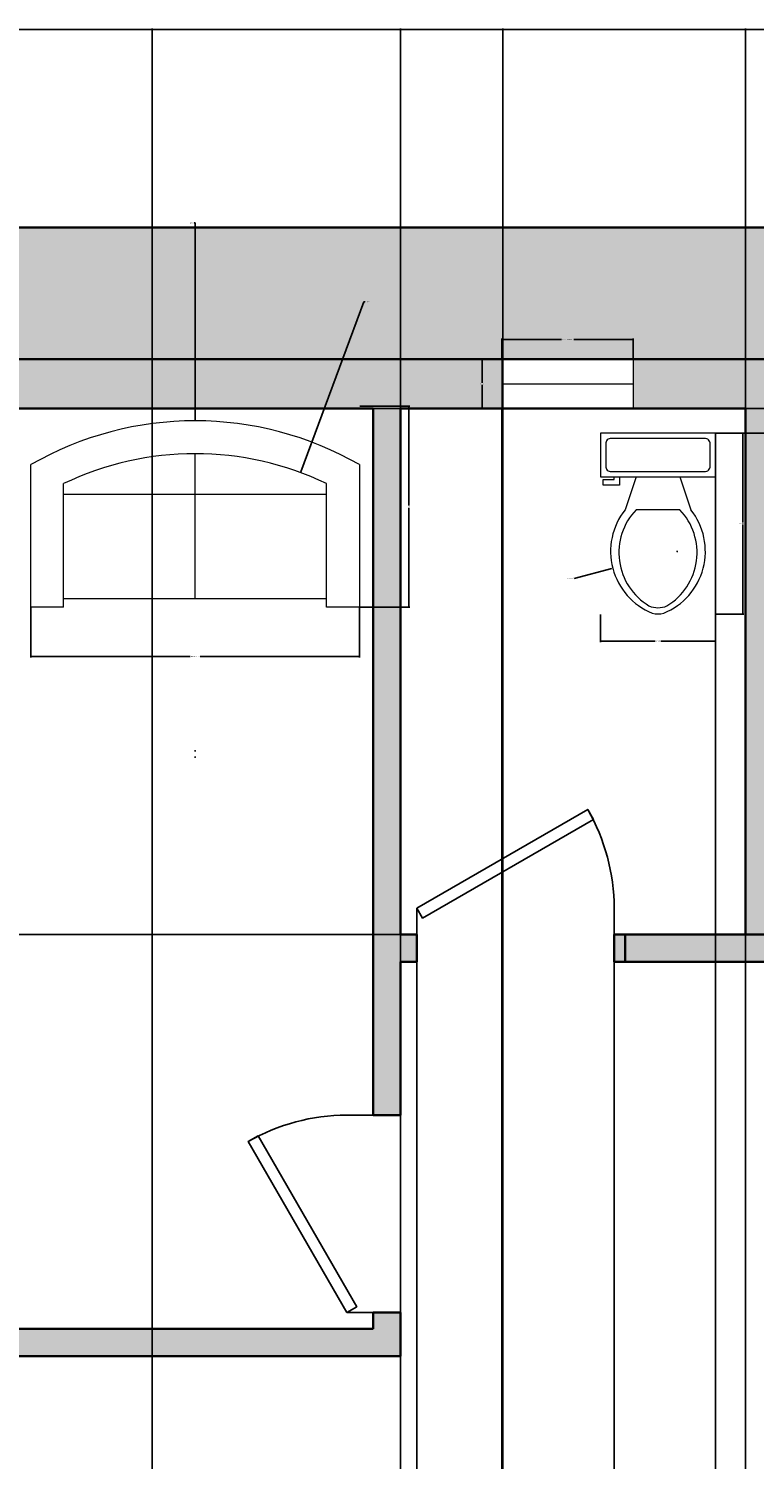
# Model space of a CAD drawing. Units: inches. Extents: x -7 to 546, y -27 to 766.
# Tile 7 of 9: x 143 to 276, y 505 to 766. Entities that reach past the tile are written whole.
import ezdxf

# ---------------------------------------------------------------- set-up
doc = ezdxf.new("R2010")
doc.units = ezdxf.units.IN
doc.header["$MEASUREMENT"] = 0
for name, color, linetype, lineweight in [('A-ANNO-DIMS', 2, 'Continuous', 18), ('A-FLOR-FIXT', 9, 'Continuous', 18), ('A-WALL', 7, 'Continuous', 35), ('C-PROP', 7, 'Continuous', 35), ('doors', 40, 'Continuous', 25), ('furniture', 220, 'Continuous', 18), ('window', 30, 'Continuous', 20)]:
    doc.layers.add(name, color=color, linetype=linetype, lineweight=lineweight)
doc.layers.add('A-WALL-PATT', color=251, linetype='Continuous', lineweight=13, true_color=0x636466)
doc.layers.add('L-PLNT-PATT', color=85, linetype='Continuous', lineweight=13, true_color=0x58ba48)
doc.styles.get("Standard").update_dxf_attribs({"font": 'arial.ttf'})
doc.dimstyles.get("Standard").update_dxf_attribs({"dimtxt": 0.18, "dimasz": 0.18, "dimexe": 0.18, "dimexo": 0.0625, "dimgap": 0.09, "dimtad": 0, "dimtih": 1, "dimtoh": 1, "dimdec": 4, "dimzin": 0, "dimdsep": 46, "dimtxsty": 'Standard', "dimcen": 0.09, "dimadec": 0, "dimazin": 0, "dimtfac": 1, "dimtdec": 4, "dimtofl": 0, "dimtmove": 0, "dimatfit": 3, "dimfxl": 1, "dimtolj": 1, "dimtzin": 0, "dimarcsym": 0})

# ---------------------------------------------------------------- blocks, each defined once
blk = doc.blocks.new('*U10')
for p, q in [((0, 0), (0, -100)), ((750, 0), (750, -100))]:
    blk.add_line(p, q)
blk.add_lwpolyline([(0, 0), (649.5, 375), (671.4, 337.1), (21.9, -37.9)], close=True)
blk.add_arc((0, 0), 750, 0, 30)
blk = doc.blocks.new('Sofa - Roundback Loveseat 5 ft.')
for p, q in [((0, -32.44198), (0, -5.99998)), ((-24, -33.99998), (-24, -11.46958)), ((24.00004, -33.99998), (24.00004, -11.46958)), ((-23.9998, -13.38178), (23.99986, -13.38178)), ((-24, -32.44198), (24.00004, -32.44198))]:
    blk.add_line(p, q)
for points in [[(-24, -33.99998), (-30, -33.99998), (-30, -7.99998)], [(30.00004, -7.99998), (30.00004, -33.99998), (24.00004, -33.99998)]]:
    blk.add_lwpolyline(points)
for centre, radius, start, end in [((0, -60.24998), 60.24998, 60.13715, 119.8628), ((0, -61.38438), 55.38444, 64.32083, 115.6792)]:
    blk.add_arc(centre, radius, start, end)
blk = doc.blocks.new('Toilet - top')
for p, q in [((9.5, -6), (9.5, -2)), ((-10, -8.5), (-8, -8.5)), ((-10, -9.5), (-10, -8.5)), ((-7, -9.5), (-10, -9.5)), ((-8, -8.5), (-8, -8)), ((-7, -8), (-7, -9.5)), ((-4, -8), (-6, -14)), ((4, -8), (6, -14)), ((4, -14), (-4, -14))]:
    blk.add_line(p, q)
blk.add_lwpolyline([(10.5, -8), (10.5, 0), (-10.5, 0), (-10.5, -8)], close=True)
for points in [[(-9.5, -2), (-9.5, -6)], [(8.5, -1), (-8.5, -1)], [(-8.5, -7), (8.5, -7)]]:
    blk.add_lwpolyline(points)
for centre, radius, start, end in [((-8.62, -1.88), 0.884, 81.8699, 188.1301), ((8.62, -1.88), 0.884, 351.8699, 98.1301), ((-8.62, -6.12), 0.884, 171.8699, 278.1301), ((8.62, -6.12), 0.884, 261.8699, 8.1301), ((3.52, -21.58), 12.17, 141.4691, 247.9714), ((4.2, -21.82), 11.33, 136.3677, 238.9468), ((-3.52, -21.58), 12.17, 292.0284, 38.5307), ((-4.2, -21.82), 11.33, 301.053, 43.6321), ((0, -27.88), 4, 245.7318, 294.2682), ((0, -29), 4, 254.8605, 285.1395)]:
    blk.add_arc(centre, radius, start, end)
blk = doc.blocks.new('WIN-24IN')
for p, q in [((0, 9), (0, 0)), ((24, 9), (0, 9)), ((0, 9), (0, 4.5)), ((24, 0), (24, 9)), ((0, 4.5), (24, 4.5)), ((0, 0), (24, 0))]:
    blk.add_line(p, q)
blk = doc.blocks.new('*D16')
at = {"layer": 'A-ANNO-DIMS', "color": 0, "lineweight": -2, "transparency": 16777216}
for p, q in [((229.74, 705.81), (229.74, 709.52)), ((229.92, 709.34), (240.62, 709.34)), ((253.56, 709.34), (242.86, 709.34)), ((253.74, 705.81), (253.74, 709.52))]:
    blk.add_line(p, q, dxfattribs=at)
at = {"layer": 'A-ANNO-DIMS', "color": 0, "transparency": 16777216}
for points in [[(229.92, 709.37), (229.92, 709.31), (229.74, 709.34)], [(253.56, 709.37), (253.56, 709.31), (253.74, 709.34)]]:
    blk.add_solid(points, dxfattribs=at)
at = {"layer": 'Defpoints', "color": 0, "transparency": 16777216}
for p in [(253.74, 709.34), (229.74, 705.74), (253.74, 705.74)]:
    blk.add_point(p, dxfattribs=at)
at = {"layer": 'A-ANNO-DIMS', "color": 0, "transparency": 16777216, "insert": (241.74, 709.34), "char_height": 0.18, "attachment_point": 5}
blk.add_mtext('\\A1;WINDOW 24 TYP.', dxfattribs=at)
blk = doc.blocks.new('*D17')
at = {"layer": 'A-ANNO-DIMS', "color": 0, "lineweight": -2, "transparency": 16777216}
for p, q in [((229.68, 705.74), (225.96, 705.74)), ((226.14, 705.56), (226.14, 701.43)), ((226.14, 696.92), (226.14, 701.06)), ((229.68, 696.74), (225.96, 696.74))]:
    blk.add_line(p, q, dxfattribs=at)
at = {"layer": 'A-ANNO-DIMS', "color": 0, "transparency": 16777216}
for points in [[(226.11, 705.56), (226.17, 705.56), (226.14, 705.74)], [(226.11, 696.92), (226.17, 696.92), (226.14, 696.74)]]:
    blk.add_solid(points, dxfattribs=at)
at = {"layer": 'Defpoints', "color": 0, "transparency": 16777216}
for p in [(226.14, 705.74), (229.74, 705.74), (229.74, 696.74)]:
    blk.add_point(p, dxfattribs=at)
at = {"layer": 'A-ANNO-DIMS', "color": 0, "transparency": 16777216, "insert": (226.14, 701.24), "char_height": 0.18, "attachment_point": 5}
blk.add_mtext('\\A1;9 TYP.', dxfattribs=at)
blk = doc.blocks.new('*D22')
at = {"layer": 'A-ANNO-DIMS', "color": 0, "lineweight": -2, "transparency": 16777216}
for p, q in [((143.76, 660.41), (143.76, 651.29)), ((203.76, 660.41), (203.76, 651.29)), ((143.94, 651.47), (172.85, 651.47)), ((203.58, 651.47), (174.67, 651.47))]:
    blk.add_line(p, q, dxfattribs=at)
at = {"layer": 'A-ANNO-DIMS', "color": 0, "transparency": 16777216}
for points in [[(143.94, 651.5), (143.94, 651.44), (143.76, 651.47)], [(203.58, 651.5), (203.58, 651.44), (203.76, 651.47)]]:
    blk.add_solid(points, dxfattribs=at)
at = {"layer": 'Defpoints', "color": 0, "transparency": 16777216}
for p in [(143.76, 660.47), (203.76, 660.47), (203.76, 651.47)]:
    blk.add_point(p, dxfattribs=at)
at = {"layer": 'A-ANNO-DIMS', "color": 0, "transparency": 16777216, "insert": (173.76, 651.47), "char_height": 0.18, "attachment_point": 5}
blk.add_mtext('\\A1;LOVESEAT 60', dxfattribs=at)
blk = doc.blocks.new('*D23')
at = {"layer": 'A-ANNO-DIMS', "color": 0, "lineweight": -2, "transparency": 16777216}
for p, q in [((203.82, 697.14), (212.94, 697.14)), ((212.76, 696.96), (212.76, 678.99)), ((212.76, 660.65), (212.76, 678.62)), ((203.82, 660.47), (212.94, 660.47))]:
    blk.add_line(p, q, dxfattribs=at)
at = {"layer": 'A-ANNO-DIMS', "color": 0, "transparency": 16777216}
for points in [[(212.73, 696.96), (212.79, 696.96), (212.76, 697.14)], [(212.73, 660.65), (212.79, 660.65), (212.76, 660.47)]]:
    blk.add_solid(points, dxfattribs=at)
at = {"layer": 'Defpoints', "color": 0, "transparency": 16777216}
for p in [(203.76, 697.14), (212.76, 697.14), (203.76, 660.47)]:
    blk.add_point(p, dxfattribs=at)
at = {"layer": 'A-ANNO-DIMS', "color": 0, "transparency": 16777216, "insert": (212.76, 678.81), "char_height": 0.18, "attachment_point": 5}
blk.add_mtext('\\A1;37', dxfattribs=at)
blk = doc.blocks.new('*D28')
at = {"layer": 'A-ANNO-DIMS', "color": 0, "lineweight": -2, "transparency": 16777216}
for p, q in [((268.8, 692.23), (273.88, 692.23)), ((273.7, 692.05), (273.7, 675.89)), ((273.7, 659.37), (273.7, 675.53)), ((268.8, 659.19), (273.88, 659.19))]:
    blk.add_line(p, q, dxfattribs=at)
at = {"layer": 'A-ANNO-DIMS', "color": 0, "transparency": 16777216}
for points in [[(273.67, 692.05), (273.73, 692.05), (273.7, 692.23)], [(273.67, 659.37), (273.73, 659.37), (273.7, 659.19)]]:
    blk.add_solid(points, dxfattribs=at)
at = {"layer": 'Defpoints', "color": 0, "transparency": 16777216}
for p in [(268.74, 692.23), (273.7, 692.23), (268.74, 659.19)]:
    blk.add_point(p, dxfattribs=at)
at = {"layer": 'A-ANNO-DIMS', "color": 0, "transparency": 16777216, "insert": (273.7, 675.71), "char_height": 0.18, "attachment_point": 5}
blk.add_mtext('\\A1;WC 33 TYP.', dxfattribs=at)
blk = doc.blocks.new('*D29')
at = {"layer": 'A-ANNO-DIMS', "color": 0, "lineweight": -2, "transparency": 16777216}
for p, q in [((247.74, 659.12), (247.74, 654.05)), ((268.74, 659.12), (268.74, 654.05)), ((247.92, 654.23), (257.71, 654.23)), ((268.56, 654.23), (258.77, 654.23))]:
    blk.add_line(p, q, dxfattribs=at)
at = {"layer": 'A-ANNO-DIMS', "color": 0, "transparency": 16777216}
for points in [[(247.92, 654.26), (247.92, 654.2), (247.74, 654.23)], [(268.56, 654.26), (268.56, 654.2), (268.74, 654.23)]]:
    blk.add_solid(points, dxfattribs=at)
at = {"layer": 'Defpoints', "color": 0, "transparency": 16777216}
for p in [(247.74, 659.19), (268.74, 659.19), (268.74, 654.23)]:
    blk.add_point(p, dxfattribs=at)
at = {"layer": 'A-ANNO-DIMS', "color": 0, "transparency": 16777216, "insert": (258.24, 654.23), "char_height": 0.18, "attachment_point": 5}
blk.add_mtext('\\A1;21 TYP.', dxfattribs=at)
blk = doc.blocks.new('*D32')
at = {"layer": 'A-ANNO-DIMS', "color": 0, "lineweight": -2, "transparency": 16777216}
for p, q in [((53.23, 705.81), (53.23, 766.05)), ((53.41, 765.87), (268.94, 765.87)), ((485.05, 765.87), (269.52, 765.87)), ((485.23, 705.81), (485.23, 766.05))]:
    blk.add_line(p, q, dxfattribs=at)
at = {"layer": 'A-ANNO-DIMS', "color": 0, "transparency": 16777216}
for points in [[(53.41, 765.9), (53.41, 765.84), (53.23, 765.87)], [(485.05, 765.9), (485.05, 765.84), (485.23, 765.87)]]:
    blk.add_solid(points, dxfattribs=at)
at = {"layer": 'Defpoints', "color": 0, "transparency": 16777216}
for p in [(485.23, 765.87), (53.23, 705.74), (485.23, 705.74)]:
    blk.add_point(p, dxfattribs=at)
at = {"layer": 'A-ANNO-DIMS', "color": 0, "transparency": 16777216, "insert": (269.23, 765.87), "char_height": 0.18, "attachment_point": 5}
blk.add_mtext('\\A1;432', dxfattribs=at)
blk = doc.blocks.new('*D36')
at = {"layer": 'A-ANNO-DIMS', "color": 0, "lineweight": -2, "transparency": 16777216}
for p, q in [((211.23, 696.81), (211.23, 766.05)), ((211.41, 765.87), (242.51, 765.87)), ((274.05, 765.87), (242.95, 765.87)), ((274.23, 696.81), (274.23, 766.05))]:
    blk.add_line(p, q, dxfattribs=at)
at = {"layer": 'A-ANNO-DIMS', "color": 0, "transparency": 16777216}
for points in [[(211.41, 765.9), (211.41, 765.84), (211.23, 765.87)], [(274.05, 765.9), (274.05, 765.84), (274.23, 765.87)]]:
    blk.add_solid(points, dxfattribs=at)
at = {"layer": 'Defpoints', "color": 0, "transparency": 16777216}
for p in [(274.23, 765.87), (211.23, 696.74), (274.23, 696.74)]:
    blk.add_point(p, dxfattribs=at)
at = {"layer": 'A-ANNO-DIMS', "color": 0, "transparency": 16777216, "insert": (242.73, 765.87), "char_height": 0.18, "attachment_point": 5}
blk.add_mtext('\\A1;63', dxfattribs=at)
blk = doc.blocks.new('*D38')
at = {"layer": 'A-ANNO-DIMS', "color": 0, "lineweight": -2, "transparency": 16777216}
for p, q in [((211.17, 696.74), (-7.07, 696.74)), ((-6.89, 696.56), (-6.89, 648.93)), ((-6.89, 600.92), (-6.89, 648.56)), ((211.17, 600.74), (-7.07, 600.74))]:
    blk.add_line(p, q, dxfattribs=at)
at = {"layer": 'A-ANNO-DIMS', "color": 0, "transparency": 16777216}
for points in [[(-6.92, 696.56), (-6.86, 696.56), (-6.89, 696.74)], [(-6.92, 600.92), (-6.86, 600.92), (-6.89, 600.74)]]:
    blk.add_solid(points, dxfattribs=at)
at = {"layer": 'Defpoints', "color": 0, "transparency": 16777216}
for p in [(211.23, 696.74), (-6.89, 600.74), (211.23, 600.74)]:
    blk.add_point(p, dxfattribs=at)
at = {"layer": 'A-ANNO-DIMS', "color": 0, "transparency": 16777216, "insert": (-6.89, 648.74), "char_height": 0.18, "attachment_point": 5}
blk.add_mtext('\\A1;96', dxfattribs=at)
blk = doc.blocks.new('*D39')
at = {"layer": 'A-ANNO-DIMS', "color": 0, "lineweight": -2, "transparency": 16777216}
for p, q in [((214.23, 600.68), (214.23, -26.56)), ((250.23, 600.68), (250.23, -26.56)), ((214.41, -26.38), (232.01, -26.38)), ((250.05, -26.38), (232.45, -26.38))]:
    blk.add_line(p, q, dxfattribs=at)
at = {"layer": 'A-ANNO-DIMS', "color": 0, "transparency": 16777216}
for points in [[(214.41, -26.35), (214.41, -26.41), (214.23, -26.38)], [(250.05, -26.35), (250.05, -26.41), (250.23, -26.38)]]:
    blk.add_solid(points, dxfattribs=at)
at = {"layer": 'Defpoints', "color": 0, "transparency": 16777216}
for p in [(214.23, 600.74), (250.23, 600.74), (250.23, -26.38)]:
    blk.add_point(p, dxfattribs=at)
at = {"layer": 'A-ANNO-DIMS', "color": 0, "transparency": 16777216, "insert": (232.23, -26.38), "char_height": 0.18, "attachment_point": 5}
blk.add_mtext('\\A1;36', dxfattribs=at)
blk = doc.blocks.new('*D41')
at = {"layer": 'A-ANNO-DIMS', "color": 0, "lineweight": -2, "transparency": 16777216}
for p, q in [((274.23, 600.68), (274.23, -26.56)), ((279.23, 600.68), (279.23, -26.56)), ((274.41, -26.38), (276.58, -26.38)), ((279.05, -26.38), (276.88, -26.38))]:
    blk.add_line(p, q, dxfattribs=at)
at = {"layer": 'A-ANNO-DIMS', "color": 0, "transparency": 16777216}
for points in [[(274.41, -26.35), (274.41, -26.41), (274.23, -26.38)], [(279.05, -26.35), (279.05, -26.41), (279.23, -26.38)]]:
    blk.add_solid(points, dxfattribs=at)
at = {"layer": 'Defpoints', "color": 0, "transparency": 16777216}
for p in [(274.23, 600.74), (279.23, 600.74), (279.23, -26.38)]:
    blk.add_point(p, dxfattribs=at)
at = {"layer": 'A-ANNO-DIMS', "color": 0, "transparency": 16777216, "insert": (276.73, -26.38), "char_height": 0.18, "attachment_point": 5}
blk.add_mtext('\\A1;5', dxfattribs=at)
blk = doc.blocks.new('*D42')
at = {"layer": 'A-ANNO-DIMS', "color": 0, "lineweight": -2, "transparency": 16777216}
for p, q in [((211.23, 696.68), (211.23, -26.56)), ((229.74, 696.68), (229.74, -26.56)), ((211.41, -26.38), (220.12, -26.38)), ((229.56, -26.38), (220.85, -26.38))]:
    blk.add_line(p, q, dxfattribs=at)
at = {"layer": 'A-ANNO-DIMS', "color": 0, "transparency": 16777216}
for points in [[(211.41, -26.35), (211.41, -26.41), (211.23, -26.38)], [(229.56, -26.35), (229.56, -26.41), (229.74, -26.38)]]:
    blk.add_solid(points, dxfattribs=at)
at = {"layer": 'Defpoints', "color": 0, "transparency": 16777216}
for p in [(211.23, 696.74), (229.74, 696.74), (229.74, -26.38)]:
    blk.add_point(p, dxfattribs=at)
at = {"layer": 'A-ANNO-DIMS', "color": 0, "transparency": 16777216, "insert": (220.49, -26.38), "char_height": 0.18, "attachment_point": 5}
blk.add_mtext('\\A1;18.51', dxfattribs=at)
blk = doc.blocks.new('*D45')
at = {"layer": 'A-ANNO-DIMS', "color": 0, "lineweight": -2, "transparency": 16777216}
for p, q in [((211.23, 600.68), (211.23, -26.56)), ((214.23, 600.68), (214.23, -26.56)), ((211.41, -26.38), (212.58, -26.38)), ((214.05, -26.38), (212.88, -26.38))]:
    blk.add_line(p, q, dxfattribs=at)
at = {"layer": 'A-ANNO-DIMS', "color": 0, "transparency": 16777216}
for points in [[(211.41, -26.35), (211.41, -26.41), (211.23, -26.38)], [(214.05, -26.35), (214.05, -26.41), (214.23, -26.38)]]:
    blk.add_solid(points, dxfattribs=at)
at = {"layer": 'Defpoints', "color": 0, "transparency": 16777216}
for p in [(211.23, 600.74), (214.23, 600.74), (214.23, -26.38)]:
    blk.add_point(p, dxfattribs=at)
at = {"layer": 'A-ANNO-DIMS', "color": 0, "transparency": 16777216, "insert": (212.73, -26.38), "char_height": 0.18, "attachment_point": 5}
blk.add_mtext('\\A1;3', dxfattribs=at)
blk = doc.blocks.new('*D53')
at = {"layer": 'A-ANNO-DIMS', "color": 0, "lineweight": -2, "transparency": 16777216}
for p, q in [((133.93, 124.01), (133.93, 766.05)), ((134.11, 765.87), (181.71, 765.87)), ((229.75, 765.87), (182.15, 765.87)), ((229.93, 124.01), (229.93, 766.05))]:
    blk.add_line(p, q, dxfattribs=at)
at = {"layer": 'A-ANNO-DIMS', "color": 0, "transparency": 16777216}
for points in [[(134.11, 765.9), (134.11, 765.84), (133.93, 765.87)], [(229.75, 765.9), (229.75, 765.84), (229.93, 765.87)]]:
    blk.add_solid(points, dxfattribs=at)
at = {"layer": 'Defpoints', "color": 0, "transparency": 16777216}
for p in [(229.93, 765.87), (133.93, 123.94), (229.93, 123.94)]:
    blk.add_point(p, dxfattribs=at)
at = {"layer": 'A-ANNO-DIMS', "color": 0, "transparency": 16777216, "insert": (181.93, 765.87), "char_height": 0.18, "attachment_point": 5}
blk.add_mtext('\\A1;96', dxfattribs=at)
blk = doc.blocks.new('*D68')
at = {"layer": 'A-ANNO-DIMS', "color": 0, "lineweight": -2, "transparency": 16777216}
for p, q in [((133.93, 100.01), (133.93, 766.05)), ((134.11, 765.87), (149.71, 765.87)), ((165.75, 765.87), (150.15, 765.87)), ((165.93, 104.01), (165.93, 766.05))]:
    blk.add_line(p, q, dxfattribs=at)
at = {"layer": 'A-ANNO-DIMS', "color": 0, "transparency": 16777216}
for points in [[(134.11, 765.9), (134.11, 765.84), (133.93, 765.87)], [(165.75, 765.9), (165.75, 765.84), (165.93, 765.87)]]:
    blk.add_solid(points, dxfattribs=at)
at = {"layer": 'Defpoints', "color": 0, "transparency": 16777216}
for p in [(165.93, 765.87), (165.93, 103.94), (133.93, 99.94)]:
    blk.add_point(p, dxfattribs=at)
at = {"layer": 'A-ANNO-DIMS', "color": 0, "transparency": 16777216, "insert": (149.93, 765.87), "char_height": 0.18, "attachment_point": 5}
blk.add_mtext('\\A1;32', dxfattribs=at)
blk = doc.blocks.new('*D81')
at = {"layer": 'A-ANNO-DIMS', "color": 0, "lineweight": -2, "transparency": 16777216}
for p, q in [((62.23, 240.81), (62.23, 766.05)), ((62.41, 765.87), (194.44, 765.87)), ((327.05, 765.87), (195.02, 765.87)), ((327.23, 234.81), (327.23, 766.05))]:
    blk.add_line(p, q, dxfattribs=at)
at = {"layer": 'A-ANNO-DIMS', "color": 0, "transparency": 16777216}
for points in [[(62.41, 765.9), (62.41, 765.84), (62.23, 765.87)], [(327.05, 765.9), (327.05, 765.84), (327.23, 765.87)]]:
    blk.add_solid(points, dxfattribs=at)
at = {"layer": 'Defpoints', "color": 0, "transparency": 16777216}
for p in [(327.23, 765.87), (62.23, 240.74), (327.23, 234.74)]:
    blk.add_point(p, dxfattribs=at)
at = {"layer": 'A-ANNO-DIMS', "color": 0, "transparency": 16777216, "insert": (194.73, 765.87), "char_height": 0.18, "attachment_point": 5}
blk.add_mtext('\\A1;265', dxfattribs=at)
blk = doc.blocks.new('*D85')
at = {"layer": 'A-ANNO-DIMS', "color": 0, "lineweight": -2, "transparency": 16777216}
for p, q in [((274.23, 696.68), (274.23, -26.56)), ((268.74, 692.17), (268.74, -26.56)), ((268.92, -26.38), (271.09, -26.38)), ((274.05, -26.38), (271.88, -26.38))]:
    blk.add_line(p, q, dxfattribs=at)
at = {"layer": 'A-ANNO-DIMS', "color": 0, "transparency": 16777216}
for points in [[(268.92, -26.35), (268.92, -26.41), (268.74, -26.38)], [(274.05, -26.35), (274.05, -26.41), (274.23, -26.38)]]:
    blk.add_solid(points, dxfattribs=at)
at = {"layer": 'Defpoints', "color": 0, "transparency": 16777216}
for p in [(274.23, 696.74), (268.74, 692.23), (268.74, -26.38)]:
    blk.add_point(p, dxfattribs=at)
at = {"layer": 'A-ANNO-DIMS', "color": 0, "transparency": 16777216, "insert": (271.49, -26.38), "char_height": 0.18, "attachment_point": 5}
blk.add_mtext('\\A1;5.493', dxfattribs=at)
blk = doc.blocks.new('*D86')
at = {"layer": 'A-ANNO-DIMS', "color": 0, "lineweight": -2, "transparency": 16777216}
for p, q in [((274.29, 696.74), (545.54, 696.74)), ((545.36, 696.56), (545.36, 694.67)), ((268.8, 692.23), (545.54, 692.23)), ((545.36, 692.41), (545.36, 694.31))]:
    blk.add_line(p, q, dxfattribs=at)
at = {"layer": 'A-ANNO-DIMS', "color": 0, "transparency": 16777216}
for points in [[(545.33, 696.56), (545.39, 696.56), (545.36, 696.74)], [(545.33, 692.41), (545.39, 692.41), (545.36, 692.23)]]:
    blk.add_solid(points, dxfattribs=at)
at = {"layer": 'Defpoints', "color": 0, "transparency": 16777216}
for p in [(274.23, 696.74), (268.74, 692.23), (545.36, 692.23)]:
    blk.add_point(p, dxfattribs=at)
at = {"layer": 'A-ANNO-DIMS', "color": 0, "transparency": 16777216, "insert": (545.36, 694.49), "char_height": 0.18, "attachment_point": 5}
blk.add_mtext('\\A1;4.512', dxfattribs=at)
blk = doc.blocks.new('*D91')
at = {"layer": 'A-ANNO-DIMS', "color": 0, "lineweight": -2, "transparency": 16777216}
for p, q in [((173.58, 730.62), (173.76, 730.62)), ((173.76, 730.62), (173.76, 694.65)), ((173.67, 634.22), (173.85, 634.22)), ((173.76, 634.13), (173.76, 634.31))]:
    blk.add_line(p, q, dxfattribs=at)
at = {"layer": 'A-ANNO-DIMS', "color": 0, "transparency": 16777216}
blk.add_solid([(173.79, 694.65), (173.73, 694.65), (173.76, 694.47)], dxfattribs=at)
at = {"layer": 'Defpoints', "color": 0, "transparency": 16777216}
for p in [(173.76, 694.47), (173.76, 634.22)]:
    blk.add_point(p, dxfattribs=at)
at = {"layer": 'A-ANNO-DIMS', "color": 0, "transparency": 16777216, "insert": (173.1, 730.62), "char_height": 0.18, "attachment_point": 5}
blk.add_mtext('\\A1;R60.25', dxfattribs=at)
blk = doc.blocks.new('*D92')
at = {"layer": 'A-ANNO-DIMS', "color": 0, "lineweight": -2, "transparency": 16777216}
for p, q in [((204.55, 716.18), (193.06, 685.19)), ((204.73, 716.18), (204.55, 716.18)), ((173.67, 633.09), (173.85, 633.09)), ((173.76, 633), (173.76, 633.18))]:
    blk.add_line(p, q, dxfattribs=at)
at = {"layer": 'A-ANNO-DIMS', "color": 0, "transparency": 16777216}
blk.add_solid([(193.04, 685.2), (193.09, 685.18), (193, 685.02)], dxfattribs=at)
at = {"layer": 'Defpoints', "color": 0, "transparency": 16777216}
for p in [(193, 685.02), (173.76, 633.09)]:
    blk.add_point(p, dxfattribs=at)
at = {"layer": 'A-ANNO-DIMS', "color": 0, "transparency": 16777216, "insert": (205.21, 716.18), "char_height": 0.18, "attachment_point": 5}
blk.add_mtext('\\A1;R55.38', dxfattribs=at)
blk = doc.blocks.new('*D93')
at = {"layer": 'A-ANNO-DIMS', "color": 0, "lineweight": -2, "transparency": 16777216}
for p, q in [((261.67, 670.65), (261.85, 670.65)), ((261.76, 670.56), (261.76, 670.74)), ((242.93, 665.71), (249.81, 667.51))]:
    blk.add_line(p, q, dxfattribs=at)
at = {"layer": 'A-ANNO-DIMS', "color": 0, "transparency": 16777216}
blk.add_solid([(249.81, 667.54), (249.82, 667.49), (249.99, 667.56)], dxfattribs=at)
at = {"layer": 'Defpoints', "color": 0, "transparency": 16777216}
for p in [(261.76, 670.65), (249.99, 667.56)]:
    blk.add_point(p, dxfattribs=at)
at = {"layer": 'A-ANNO-DIMS', "color": 0, "transparency": 16777216, "insert": (242.25, 665.71), "char_height": 0.18, "attachment_point": 5}
blk.add_mtext('\\A1;6X R12.17', dxfattribs=at)

msp = doc.modelspace()

# ---------------------------------------------------------------- hatches: boundary and pattern name
at = {"layer": 'A-WALL-PATT'}
h = msp.add_hatch(color=256, dxfattribs=at)
h.dxf.hatch_style = 1
h.paths.add_polyline_path([(62.2319, 696.744), (86.6896, 696.744), (86.6896, 705.744), (53.2319, 705.744), (53.2319, 627.8642), (57.7271, 627.8642), (62.2319, 627.8642)])
h.paths.add_polyline_path([(229.7414, 705.744), (134.6896, 705.744), (134.6896, 696.744), (206.2319, 696.744), (206.2319, 567.744), (211.2319, 567.744), (211.2319, 595.744), (214.2319, 595.744), (214.2319, 600.744), (211.2319, 600.744), (211.2319, 696.744), (229.7414, 696.744)])
h.paths.add_polyline_path([(293.8423, 705.744), (253.7414, 705.744), (253.7414, 696.744), (274.2319, 696.744), (274.2319, 600.744), (279.2319, 600.744), (279.2319, 696.744), (293.8423, 696.744)])
h.paths.add_polyline_path([(393.9743, 705.744), (317.8423, 705.744), (317.8423, 696.744), (327.2319, 696.744), (327.2319, 651.744), (332.2319, 651.744), (332.2319, 696.744), (393.9743, 696.744)])
h.paths.add_polyline_path([(485.2319, 705.744), (441.9743, 705.744), (441.9743, 696.744), (476.2319, 696.744), (476.2319, 663.6898), (480.7319, 663.6898), (485.2319, 663.6898)])
h.paths.add_polyline_path([(485.2319, 615.6898), (476.2319, 615.6898), (476.2319, 528.744), (332.2319, 528.744), (332.2319, 531.744), (327.2319, 531.744), (327.2319, 523.744), (375.2319, 523.744), (375.2319, 427.744), (327.2319, 427.744), (327.2319, 419.744), (332.2319, 419.744), (332.2319, 422.744), (413.089, 422.744), (413.089, 427.744), (380.2319, 427.744), (380.2319, 523.744), (476.2319, 523.744), (476.2319, 490.9334), (485.2319, 490.9334)])
h.paths.add_polyline_path([(485.2319, 466.9334), (476.2319, 466.9334), (476.2319, 370.0932), (480.7319, 370.0932), (485.2319, 370.0932)])
h.paths.add_polyline_path([(485.2319, 322.0932), (476.2319, 322.0932), (476.2319, 278.744), (332.2319, 278.744), (332.2319, 383.744), (327.2319, 383.744), (327.2319, 273.744), (327.2319, 270.744), (332.2319, 270.744), (332.2319, 273.744), (476.2319, 273.744), (476.2319, 201.0338), (480.7319, 201.0338), (485.2319, 201.0338)])
h.paths.add_polyline_path([(485.2319, 153.0338), (476.2319, 153.0338), (476.2319, 42.744), (461.2319, 42.744), (461.2319, 33.744), (485.2319, 33.744)])
h.paths.add_polyline_path([(332.2319, 234.744), (327.2319, 234.744), (327.2319, 160.744), (315.2319, 160.744), (315.2319, 151.744), (327.2319, 151.744), (327.2319, 33.744), (332.2319, 33.744)])
h.paths.add_polyline_path([(252.2319, 151.744), (258.4464, 151.744), (264.2319, 151.744), (264.2319, 160.744), (252.2319, 160.744), (252.2319, 172.744), (247.2319, 172.744), (247.2319, 91.744), (127.2319, 91.744), (127.2319, 196.744), (122.2319, 196.744), (122.2319, 91.744), (62.2319, 91.744), (62.2319, 126.1124), (53.2319, 126.1124), (53.2319, 9.744), (62.2319, 9.744), (62.2319, 86.744), (247.2319, 86.744), (247.2319, 33.744), (252.2319, 33.744), (252.2319, 53.744)])
h.paths.add_polyline_path([(62.2319, 235.744), (122.2319, 235.744), (122.2319, 232.744), (127.2319, 232.744), (127.2319, 235.744), (247.2319, 235.744), (247.2319, 220.744), (252.2319, 220.744), (252.2319, 240.744), (250.6678, 240.744), (247.2319, 240.744), (62.2319, 240.744), (62.2319, 322.0932), (53.2319, 322.0932), (53.2319, 174.1124), (57.7271, 174.1124), (62.2319, 174.1124)])
h = msp.add_hatch(color=256, dxfattribs=at)
h.dxf.hatch_style = 1
h.paths.add_polyline_path([(327.2319, 600.744), (252.2319, 600.744), (252.2319, 595.744), (327.2319, 595.744)])
h.paths.add_polyline_path([(332.2319, 615.744), (327.2319, 615.744), (327.2319, 567.744), (332.2319, 567.744)])
h.paths.add_polyline_path([(252.2319, 600.744), (250.2319, 600.744), (250.2319, 595.744), (252.2319, 595.744)])
h = msp.add_hatch(color=256, dxfattribs=at)
h.dxf.hatch_style = 1
h.paths.add_polyline_path([(62.2319, 456.9275), (53.2319, 456.9275), (53.2319, 370.0932), (57.7271, 370.0932), (62.2319, 370.0932)])
h.paths.add_polyline_path([(62.2319, 579.8642), (53.2319, 579.8642), (53.2319, 504.9275), (57.7271, 504.9275), (62.2319, 504.9275), (62.2319, 523.744), (211.2319, 523.744), (211.2319, 531.744), (206.2319, 531.744), (206.2319, 528.744), (62.2319, 528.744)])
at = {"layer": 'L-PLNT-PATT'}
h = msp.add_hatch(color=256, dxfattribs=at)
h.dxf.hatch_style = 1
h.paths.add_polyline_path([(509.2319, 729.744), (29.2319, 729.744), (29.2319, 9.744), (53.2319, 9.744), (53.2319, 705.744), (485.2319, 705.744), (485.2319, 33.744), (461.2319, 33.744), (461.2319, 9.744), (509.2319, 9.744)])

# ---------------------------------------------------------------- linework, layer by layer
at = {"layer": 'A-WALL'}
for p, q in [((206.2319, 696.744), (62.2319, 696.744)), ((206.2319, 696.744), (206.2319, 567.744)), ((274.2319, 696.744), (211.2319, 696.744)), ((211.2319, 696.744), (211.2319, 600.744)), ((274.2319, 600.744), (274.2319, 696.744)), ((214.2319, 600.744), (211.2319, 600.744)), ((214.2319, 600.744), (214.2319, 595.744)), ((327.2319, 600.744), (250.2319, 600.744)), ((250.2319, 600.744), (250.2319, 595.744)), ((252.2319, 600.744), (252.2319, 595.744)), ((214.2319, 595.744), (211.2319, 595.744)), ((211.2319, 595.744), (211.2319, 567.744)), ((327.2319, 595.744), (250.2319, 595.744)), ((211.2319, 567.744), (206.2319, 567.744)), ((211.2319, 531.744), (206.2319, 531.744)), ((206.2319, 531.744), (206.2319, 528.744)), ((211.2319, 531.744), (211.2319, 523.744)), ((206.2319, 528.744), (62.2319, 528.744)), ((211.2319, 523.744), (62.2319, 523.744))]:
    msp.add_line(p, q, dxfattribs=at)
msp.add_lwpolyline([(461.2319, 33.744), (485.2319, 33.744), (485.2319, 705.744), (53.2319, 705.744), (53.2319, 9.744)], dxfattribs=at)
at = {"layer": 'C-PROP'}
msp.add_lwpolyline([(29.2319, 9.744), (509.2319, 9.744), (509.2319, 729.744), (29.2319, 729.744)], close=True, dxfattribs=at)

# ---------------------------------------------------------------- block references
at = {"layer": 'A-FLOR-FIXT'}
msp.add_blockref('Toilet - top', (258.2385, 692.2322), dxfattribs=at)
at = {"layer": 'doors', "xscale": 0.0480000000000013, "yscale": 0.0480000000000013, "zscale": 0.0480000000000013}
msp.add_blockref('*U10', (214.2319, 605.544), dxfattribs=at)
at = {"layer": 'doors', "xscale": 0.0480000000000013, "yscale": 0.0480000000000013, "zscale": 0.0480000000000013, "rotation": 90}
msp.add_blockref('*U10', (201.4319, 531.744), dxfattribs=at)
at = {"layer": 'furniture'}
msp.add_blockref('Sofa - Roundback Loveseat 5 ft.', (173.7595, 694.4717), dxfattribs=at)
at = {"layer": 'window'}
msp.add_blockref('WIN-24IN', (229.741, 696.744), dxfattribs=at)

# ---------------------------------------------------------------- dimensions: what is measured, and where the dimension line sits
at = {"layer": 'A-ANNO-DIMS'}
for base, p1, p2, override, picture, middle in [((485.2319, 765.869), (53.2319, 705.744), (485.2319, 705.744), {"dimdec": 0, "dimlfac": 1, "dimrnd": 0, "dimzin": 0, "dimdsep": 46, "dimlunit": 2}, '*D32', (269.2319, 765.869)), ((327.2319, 765.869), (62.2319, 240.744), (327.2319, 234.744), {"dimdec": 0, "dimlfac": 1, "dimrnd": 0, "dimzin": 0, "dimdsep": 46, "dimlunit": 2}, '*D81', (194.7319, 765.869)), ((229.9271, 765.869), (133.9271, 123.9426), (229.9271, 123.9426), {"dimdec": 0, "dimlfac": 1, "dimrnd": 0, "dimzin": 0, "dimdsep": 46, "dimlunit": 2}, '*D53', (181.9271, 765.869)), ((165.9271, 765.869), (133.9271, 99.9426), (165.9271, 103.9426), {"dimdec": 0, "dimlfac": 1, "dimrnd": 0, "dimzin": 0, "dimdsep": 46, "dimlunit": 2}, '*D68', (149.9271, 765.869)), ((274.2319, 765.869), (211.2319, 696.744), (274.2319, 696.744), {"dimdec": 0, "dimlfac": 1, "dimrnd": 0, "dimzin": 0, "dimdsep": 46, "dimlunit": 2}, '*D36', (242.7319, 765.869)), ((229.7414, -26.381), (211.2319, 696.744), (229.7414, 696.744), {"dimdec": 2, "dimlfac": 1, "dimrnd": 0, "dimzin": 0, "dimdsep": 46, "dimlunit": 2}, '*D42', (220.4867, -26.381)), ((268.7385, -26.381), (274.2319, 696.744), (268.7385, 692.2322), {"dimdec": 3, "dimlfac": 1, "dimrnd": 0, "dimzin": 0, "dimdsep": 46, "dimlunit": 2}, '*D85', (271.4852, -26.381)), ((214.2319, -26.381), (211.2319, 600.744), (214.2319, 600.744), {"dimdec": 0, "dimlfac": 1, "dimrnd": 0, "dimzin": 0, "dimdsep": 46, "dimlunit": 2}, '*D45', (212.7319, -26.381)), ((250.2319, -26.381), (214.2319, 600.744), (250.2319, 600.744), {"dimdec": 0, "dimlfac": 1, "dimrnd": 0, "dimzin": 0, "dimdsep": 46, "dimlunit": 2}, '*D39', (232.2319, -26.381)), ((279.2319, -26.381), (274.2319, 600.744), (279.2319, 600.744), {"dimdec": 0, "dimlfac": 1, "dimrnd": 0, "dimzin": 0, "dimdsep": 46, "dimlunit": 2}, '*D41', (276.7319, -26.381))]:
    dim = msp.add_linear_dim(base=base, p1=p1, p2=p2, dimstyle='Standard', override=override, dxfattribs=at)
    dim.commit()
    dim.dimension.update_dxf_attribs({"geometry": picture, "text_midpoint": middle})
for center, mpoint, picture, middle in [((173.7595, 634.2217), (173.759, 694.4717), '*D91', (173.0982, 730.6217)), ((173.7595, 633.0873), (193.0007, 685.022), '*D92', (205.2055, 716.1828))]:
    dim = msp.add_radius_dim(center=center, mpoint=mpoint, dimstyle='Standard', override={"dimdec": 2, "dimlfac": 1, "dimrnd": 0, "dimzin": 0, "dimdsep": 46, "dimlunit": 2}, dxfattribs=at)
    dim.commit()
    dim.dimension.update_dxf_attribs({"geometry": picture, "text_midpoint": middle, "dimtype": 164})
for base, p1, p2, text, picture, middle in [((253.7414, 709.344), (229.7414, 705.744), (253.7414, 705.744), 'WINDOW <> TYP.', '*D16', (241.7414, 709.344)), ((203.7595, 651.4717), (143.7595, 660.4717), (203.7595, 660.4717), 'LOVESEAT <>', '*D22', (173.7595, 651.4717)), ((268.7385, 654.229), (247.7385, 659.1859), (268.7385, 659.1859), '<> TYP.', '*D29', (258.2385, 654.229))]:
    dim = msp.add_linear_dim(base=base, p1=p1, p2=p2, text=text, dimstyle='Standard', override={"dimdec": 0, "dimlfac": 1, "dimrnd": 0, "dimzin": 0, "dimdsep": 46, "dimlunit": 2}, dxfattribs=at)
    dim.commit()
    dim.dimension.update_dxf_attribs({"geometry": picture, "text_midpoint": middle})
for base, p1, p2, text, picture, middle in [((226.1414, 705.744), (229.7414, 696.744), (229.7414, 705.744), '<> TYP.', '*D17', (226.1414, 701.244)), ((273.6954, 692.2322), (268.7385, 659.1859), (268.7385, 692.2322), 'WC <> TYP.', '*D28', (273.6954, 675.7091))]:
    dim = msp.add_linear_dim(base=base, p1=p1, p2=p2, angle=90, text=text, dimstyle='Standard', override={"dimdec": 0, "dimlfac": 1, "dimrnd": 0, "dimzin": 0, "dimdsep": 46, "dimlunit": 2}, dxfattribs=at)
    dim.commit()
    dim.dimension.update_dxf_attribs({"geometry": picture, "text_midpoint": middle})
for base, p1, p2, override, picture, middle in [((-6.8931, 600.744), (211.2319, 696.744), (211.2319, 600.744), {"dimdec": 0, "dimlfac": 1, "dimrnd": 0, "dimzin": 0, "dimdsep": 46, "dimlunit": 2}, '*D38', (-6.8931, 648.744)), ((212.7595, 697.1384), (203.7595, 660.4717), (203.7595, 697.1384), {"dimdec": 0, "dimlfac": 1, "dimrnd": 0, "dimzin": 0, "dimdsep": 46, "dimlunit": 2}, '*D23', (212.7595, 678.8051)), ((545.3569, 692.2322), (274.2319, 696.744), (268.7385, 692.2322), {"dimdec": 3, "dimlfac": 1, "dimrnd": 0, "dimzin": 0, "dimdsep": 46, "dimlunit": 2}, '*D86', (545.3569, 694.4881))]:
    dim = msp.add_linear_dim(base=base, p1=p1, p2=p2, angle=90, dimstyle='Standard', override=override, dxfattribs=at)
    dim.commit()
    dim.dimension.update_dxf_attribs({"geometry": picture, "text_midpoint": middle})
dim = msp.add_radius_dim(center=(261.758, 670.6517), mpoint=(249.9883, 667.5601), text='6X <>', dimstyle='Standard', override={"dimdec": 2, "dimlfac": 1, "dimrnd": 0, "dimzin": 0, "dimdsep": 46, "dimlunit": 2}, dxfattribs=at)
dim.commit()
dim.dimension.update_dxf_attribs({"geometry": '*D93', "text_midpoint": (242.9264, 665.7051), "dimtype": 164})

doc.saveas('drawing.dxf')
